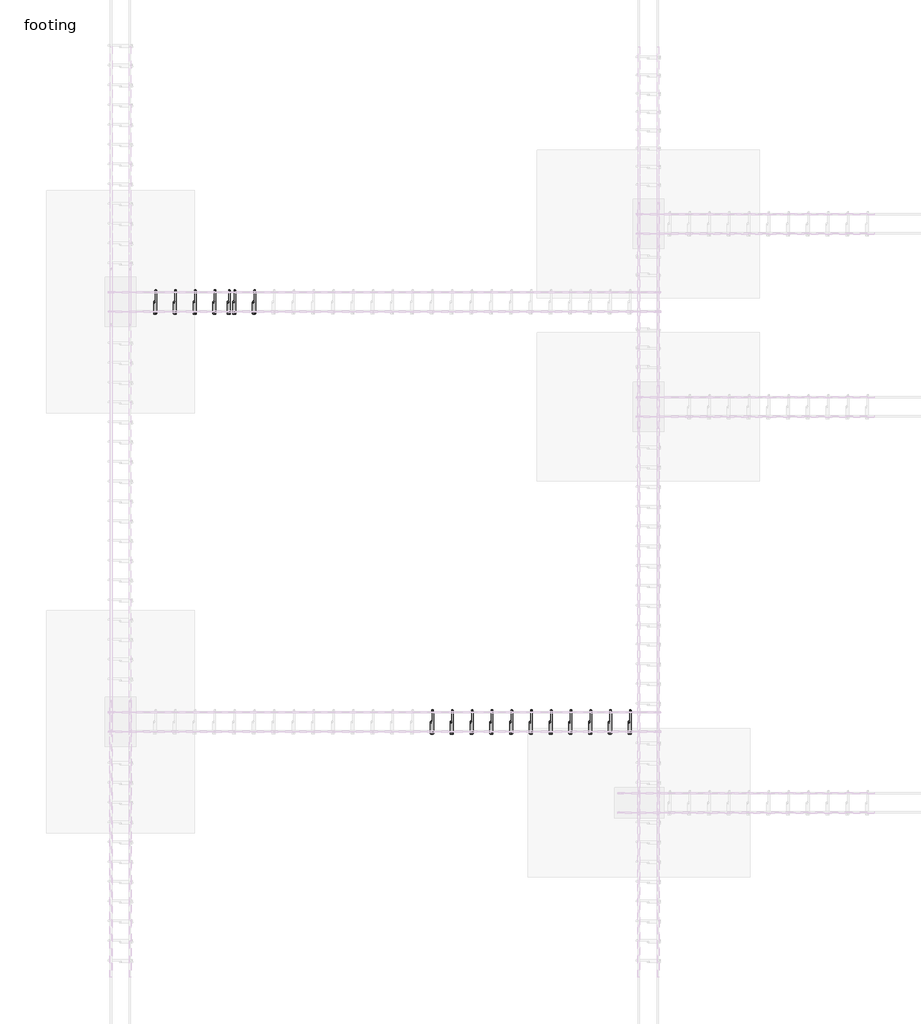
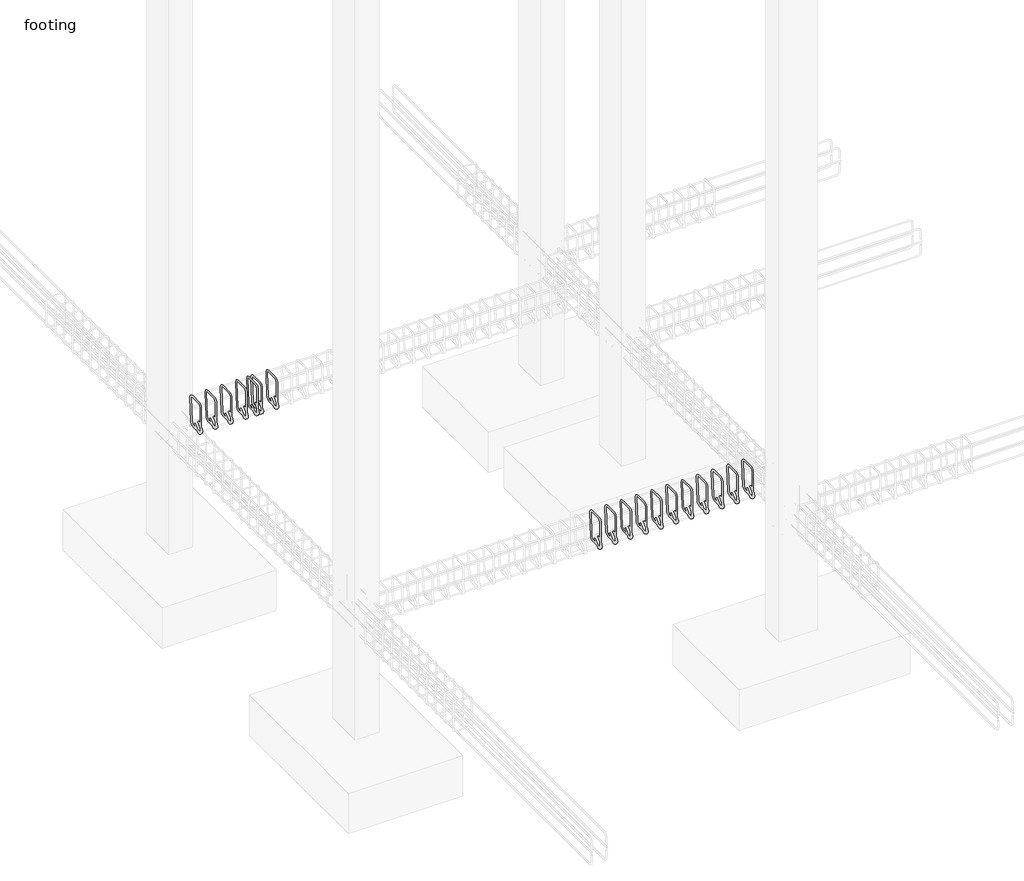
# One storey, part 7 of 21: 18 reinforcing bars.
"""IFC4 building model written with IfcOpenShell, lengths in millimetres."""

from ifc_helpers import new_model, si_unit, point, frame, origin, place, context, project, spatial, polyline, circle_curve, trimmed, segment, composite_curve, element, save
from ifc_brep_helpers import swept_disk

model = new_model("IFC4")

# Units and contexts
model_context = context("Model", 3, world=origin())
ifc_project = project(units=[si_unit("LENGTHUNIT", "METRE", prefix="MILLI")], contexts=[model_context])

# Site, building, storey
site = spatial("IfcSite", under=ifc_project)
building = spatial("IfcBuilding", under=site)
storey = spatial("IfcBuildingStorey", under=building, Name="footing", Elevation=-1524.0)

# Reinforcing bars
placement = place(None, origin())
element("IfcReinforcingBar", 1, at=placement, inside=storey, context=model_context, shape_type="SolidModel", body=[
    swept_disk(composite_curve([segment(polyline([(-9654.4883428, 4117.8887132, -310.8825168), (-9654.4883428, 4063.0237147, -365.7475153)]), True, "CONTINUOUS"), segment(trimmed(circle_curve(frame((-9654.4883428, 4040.5730744, -343.296875), z_axis=(-1.0, 0.0, 0.0), x_axis=(0.0, 22.450640299999577, -22.450640299999975)), 31.75), [point((-9654.4883428, 4063.0237147, -365.7475153))], [point((-9654.4883428, 4008.8230744, -343.296875))], True, "CARTESIAN"), True, "CONTINUOUS"), segment(polyline([(-9654.4883428, 4008.8230744, -343.296875), (-9654.4883428, 4008.8230744, -63.103125)]), True, "CONTINUOUS"), segment(trimmed(circle_curve(frame((-9654.4883428, 4040.5730744, -63.103125), z_axis=(-1.0, 0.0, 0.0), x_axis=(0.0, -31.75, 0.0)), 31.75), [point((-9654.4883428, 4008.8230744, -63.103125))], [point((-9654.4883428, 4040.5730744, -31.353125))], True, "CARTESIAN"), True, "CONTINUOUS"), segment(polyline([(-9654.4883428, 4040.5730744, -31.353125), (-9654.4883428, 4168.3668244, -31.353125)]), True, "CONTINUOUS"), segment(trimmed(circle_curve(frame((-9653.3159328, 4168.3668244, -63.0814712), z_axis=(-0.9993179916193466, 0.0, -0.03692629992126919), x_axis=(-1.1724099999992177, 0.0, 31.728346200000004)), 31.75), [point((-9654.4883428, 4168.3668244, -31.353125))], [point((-9653.3159328, 4200.1168244, -63.0814712))], True, "CARTESIAN"), True, "CONTINUOUS"), segment(polyline([(-9653.3159328, 4200.1168244, -63.0814712), (-9642.9607528, 4200.1168244, -343.3185288)]), True, "CONTINUOUS"), segment(trimmed(circle_curve(frame((-9642.9607528, 4168.3668244, -343.3185288), z_axis=(-0.9993179916193466, 0.0, -0.03692629992126919), x_axis=(0.0, 31.75, 0.0)), 31.75), [point((-9642.9607528, 4200.1168244, -343.3185288))], [point((-9641.7883428, 4168.3668244, -375.046875))], True, "CARTESIAN"), True, "CONTINUOUS"), segment(polyline([(-9641.7883428, 4168.3668244, -375.046875), (-9641.7883428, 4040.5730744, -375.046875)]), True, "CONTINUOUS"), segment(trimmed(circle_curve(frame((-9641.7883428, 4040.5730744, -343.296875), z_axis=(-1.0, 0.0, 0.0), x_axis=(0.0, 0.0, -31.75)), 31.75), [point((-9641.7883428, 4040.5730744, -375.046875))], [point((-9641.7883428, 4018.1224341, -320.8462347))], True, "CARTESIAN"), True, "CONTINUOUS"), segment(polyline([(-9641.7883428, 4018.1224341, -320.8462347), (-9641.7883428, 4072.9874326, -265.9812362)]), True, "CONTINUOUS")], self_intersect=False), 6.35),
])
element("IfcReinforcingBar", 2, at=placement, inside=storey, context=model_context, shape_type="SolidModel", body=[
    swept_disk(composite_curve([segment(polyline([(-9491.7883428, 4117.8887132, -310.8825168), (-9491.7883428, 4063.0237147, -365.7475153)]), True, "CONTINUOUS"), segment(trimmed(circle_curve(frame((-9491.7883428, 4040.5730744, -343.296875), z_axis=(-1.0, 0.0, 0.0), x_axis=(0.0, 22.450640299999577, -22.450640299999975)), 31.75), [point((-9491.7883428, 4063.0237147, -365.7475153))], [point((-9491.7883428, 4008.8230744, -343.296875))], True, "CARTESIAN"), True, "CONTINUOUS"), segment(polyline([(-9491.7883428, 4008.8230744, -343.296875), (-9491.7883428, 4008.8230744, -63.103125)]), True, "CONTINUOUS"), segment(trimmed(circle_curve(frame((-9491.7883428, 4040.5730744, -63.103125), z_axis=(-1.0, 0.0, 0.0), x_axis=(0.0, -31.75, 0.0)), 31.75), [point((-9491.7883428, 4008.8230744, -63.103125))], [point((-9491.7883428, 4040.5730744, -31.353125))], True, "CARTESIAN"), True, "CONTINUOUS"), segment(polyline([(-9491.7883428, 4040.5730744, -31.353125), (-9491.7883428, 4168.3668244, -31.353125)]), True, "CONTINUOUS"), segment(trimmed(circle_curve(frame((-9490.6159328, 4168.3668244, -63.0814712), z_axis=(-0.9993179916193466, 0.0, -0.03692629992126919), x_axis=(-1.1724100000010367, 0.0, 31.728346200000004)), 31.75), [point((-9491.7883428, 4168.3668244, -31.353125))], [point((-9490.6159328, 4200.1168244, -63.0814712))], True, "CARTESIAN"), True, "CONTINUOUS"), segment(polyline([(-9490.6159328, 4200.1168244, -63.0814712), (-9480.2607528, 4200.1168244, -343.3185288)]), True, "CONTINUOUS"), segment(trimmed(circle_curve(frame((-9480.2607528, 4168.3668244, -343.3185288), z_axis=(-0.9993179916193466, 0.0, -0.03692629992126919), x_axis=(0.0, 31.75, 0.0)), 31.75), [point((-9480.2607528, 4200.1168244, -343.3185288))], [point((-9479.0883428, 4168.3668244, -375.046875))], True, "CARTESIAN"), True, "CONTINUOUS"), segment(polyline([(-9479.0883428, 4168.3668244, -375.046875), (-9479.0883428, 4040.5730744, -375.046875)]), True, "CONTINUOUS"), segment(trimmed(circle_curve(frame((-9479.0883428, 4040.5730744, -343.296875), z_axis=(-1.0, 0.0, 0.0), x_axis=(0.0, 0.0, -31.75)), 31.75), [point((-9479.0883428, 4040.5730744, -375.046875))], [point((-9479.0883428, 4018.1224341, -320.8462347))], True, "CARTESIAN"), True, "CONTINUOUS"), segment(polyline([(-9479.0883428, 4018.1224341, -320.8462347), (-9479.0883428, 4072.9874326, -265.9812362)]), True, "CONTINUOUS")], self_intersect=False), 6.35),
])
element("IfcReinforcingBar", 3, at=placement, inside=storey, context=model_context, shape_type="SolidModel", body=[
    swept_disk(composite_curve([segment(polyline([(-9329.0883428, 4117.8887132, -310.8825168), (-9329.0883428, 4063.0237147, -365.7475153)]), True, "CONTINUOUS"), segment(trimmed(circle_curve(frame((-9329.0883428, 4040.5730744, -343.296875), z_axis=(-1.0, 0.0, 0.0), x_axis=(0.0, 22.450640299999577, -22.450640299999975)), 31.75), [point((-9329.0883428, 4063.0237147, -365.7475153))], [point((-9329.0883428, 4008.8230744, -343.296875))], True, "CARTESIAN"), True, "CONTINUOUS"), segment(polyline([(-9329.0883428, 4008.8230744, -343.296875), (-9329.0883428, 4008.8230744, -63.103125)]), True, "CONTINUOUS"), segment(trimmed(circle_curve(frame((-9329.0883428, 4040.5730744, -63.103125), z_axis=(-1.0, 0.0, 0.0), x_axis=(0.0, -31.75, 0.0)), 31.75), [point((-9329.0883428, 4008.8230744, -63.103125))], [point((-9329.0883428, 4040.5730744, -31.353125))], True, "CARTESIAN"), True, "CONTINUOUS"), segment(polyline([(-9329.0883428, 4040.5730744, -31.353125), (-9329.0883428, 4168.3668244, -31.353125)]), True, "CONTINUOUS"), segment(trimmed(circle_curve(frame((-9327.9159328, 4168.3668244, -63.0814712), z_axis=(-0.9993179916193466, 0.0, -0.03692629992126919), x_axis=(-1.1724099999992177, 0.0, 31.728346200000004)), 31.75), [point((-9329.0883428, 4168.3668244, -31.353125))], [point((-9327.9159328, 4200.1168244, -63.0814712))], True, "CARTESIAN"), True, "CONTINUOUS"), segment(polyline([(-9327.9159328, 4200.1168244, -63.0814712), (-9317.5607528, 4200.1168244, -343.3185288)]), True, "CONTINUOUS"), segment(trimmed(circle_curve(frame((-9317.5607528, 4168.3668244, -343.3185288), z_axis=(-0.9993179916193466, 0.0, -0.03692629992126919), x_axis=(0.0, 31.75, 0.0)), 31.75), [point((-9317.5607528, 4200.1168244, -343.3185288))], [point((-9316.3883428, 4168.3668244, -375.046875))], True, "CARTESIAN"), True, "CONTINUOUS"), segment(polyline([(-9316.3883428, 4168.3668244, -375.046875), (-9316.3883428, 4040.5730744, -375.046875)]), True, "CONTINUOUS"), segment(trimmed(circle_curve(frame((-9316.3883428, 4040.5730744, -343.296875), z_axis=(-1.0, 0.0, 0.0), x_axis=(0.0, 0.0, -31.75)), 31.75), [point((-9316.3883428, 4040.5730744, -375.046875))], [point((-9316.3883428, 4018.1224341, -320.8462347))], True, "CARTESIAN"), True, "CONTINUOUS"), segment(polyline([(-9316.3883428, 4018.1224341, -320.8462347), (-9316.3883428, 4072.9874326, -265.9812362)]), True, "CONTINUOUS")], self_intersect=False), 6.35),
])
element("IfcReinforcingBar", 4, at=placement, inside=storey, context=model_context, shape_type="SolidModel", body=[
    swept_disk(composite_curve([segment(polyline([(-9166.3883428, 4117.8887132, -310.8825168), (-9166.3883428, 4063.0237147, -365.7475153)]), True, "CONTINUOUS"), segment(trimmed(circle_curve(frame((-9166.3883428, 4040.5730744, -343.296875), z_axis=(-1.0, 0.0, 0.0), x_axis=(0.0, 22.450640299999577, -22.450640299999975)), 31.75), [point((-9166.3883428, 4063.0237147, -365.7475153))], [point((-9166.3883428, 4008.8230744, -343.296875))], True, "CARTESIAN"), True, "CONTINUOUS"), segment(polyline([(-9166.3883428, 4008.8230744, -343.296875), (-9166.3883428, 4008.8230744, -63.103125)]), True, "CONTINUOUS"), segment(trimmed(circle_curve(frame((-9166.3883428, 4040.5730744, -63.103125), z_axis=(-1.0, 0.0, 0.0), x_axis=(0.0, -31.75, 0.0)), 31.75), [point((-9166.3883428, 4008.8230744, -63.103125))], [point((-9166.3883428, 4040.5730744, -31.353125))], True, "CARTESIAN"), True, "CONTINUOUS"), segment(polyline([(-9166.3883428, 4040.5730744, -31.353125), (-9166.3883428, 4168.3668244, -31.353125)]), True, "CONTINUOUS"), segment(trimmed(circle_curve(frame((-9165.2159328, 4168.3668244, -63.0814712), z_axis=(-0.9993179916193466, 0.0, -0.03692629992126919), x_axis=(-1.1724100000010367, 0.0, 31.728346200000004)), 31.75), [point((-9166.3883428, 4168.3668244, -31.353125))], [point((-9165.2159328, 4200.1168244, -63.0814712))], True, "CARTESIAN"), True, "CONTINUOUS"), segment(polyline([(-9165.2159328, 4200.1168244, -63.0814712), (-9154.8607528, 4200.1168244, -343.3185288)]), True, "CONTINUOUS"), segment(trimmed(circle_curve(frame((-9154.8607528, 4168.3668244, -343.3185288), z_axis=(-0.9993179916193466, 0.0, -0.03692629992126919), x_axis=(0.0, 31.75, 0.0)), 31.75), [point((-9154.8607528, 4200.1168244, -343.3185288))], [point((-9153.6883428, 4168.3668244, -375.046875))], True, "CARTESIAN"), True, "CONTINUOUS"), segment(polyline([(-9153.6883428, 4168.3668244, -375.046875), (-9153.6883428, 4040.5730744, -375.046875)]), True, "CONTINUOUS"), segment(trimmed(circle_curve(frame((-9153.6883428, 4040.5730744, -343.296875), z_axis=(-1.0, 0.0, 0.0), x_axis=(0.0, 0.0, -31.75)), 31.75), [point((-9153.6883428, 4040.5730744, -375.046875))], [point((-9153.6883428, 4018.1224341, -320.8462347))], True, "CARTESIAN"), True, "CONTINUOUS"), segment(polyline([(-9153.6883428, 4018.1224341, -320.8462347), (-9153.6883428, 4072.9874326, -265.9812362)]), True, "CONTINUOUS")], self_intersect=False), 6.35),
])
element("IfcReinforcingBar", 5, at=placement, inside=storey, context=model_context, shape_type="SolidModel", body=[
    swept_disk(composite_curve([segment(polyline([(-9003.6883428, 4117.8887132, -310.8825168), (-9003.6883428, 4063.0237147, -365.7475153)]), True, "CONTINUOUS"), segment(trimmed(circle_curve(frame((-9003.6883428, 4040.5730744, -343.296875), z_axis=(-1.0, 0.0, 0.0), x_axis=(0.0, 22.450640299999577, -22.450640299999975)), 31.75), [point((-9003.6883428, 4063.0237147, -365.7475153))], [point((-9003.6883428, 4008.8230744, -343.296875))], True, "CARTESIAN"), True, "CONTINUOUS"), segment(polyline([(-9003.6883428, 4008.8230744, -343.296875), (-9003.6883428, 4008.8230744, -63.103125)]), True, "CONTINUOUS"), segment(trimmed(circle_curve(frame((-9003.6883428, 4040.5730744, -63.103125), z_axis=(-1.0, 0.0, 0.0), x_axis=(0.0, -31.75, 0.0)), 31.75), [point((-9003.6883428, 4008.8230744, -63.103125))], [point((-9003.6883428, 4040.5730744, -31.353125))], True, "CARTESIAN"), True, "CONTINUOUS"), segment(polyline([(-9003.6883428, 4040.5730744, -31.353125), (-9003.6883428, 4168.3668244, -31.353125)]), True, "CONTINUOUS"), segment(trimmed(circle_curve(frame((-9002.5159328, 4168.3668244, -63.0814712), z_axis=(-0.9993179916193466, 0.0, -0.03692629992126919), x_axis=(-1.1724099999992177, 0.0, 31.728346200000004)), 31.75), [point((-9003.6883428, 4168.3668244, -31.353125))], [point((-9002.5159328, 4200.1168244, -63.0814712))], True, "CARTESIAN"), True, "CONTINUOUS"), segment(polyline([(-9002.5159328, 4200.1168244, -63.0814712), (-8992.1607528, 4200.1168244, -343.3185288)]), True, "CONTINUOUS"), segment(trimmed(circle_curve(frame((-8992.1607528, 4168.3668244, -343.3185288), z_axis=(-0.9993179916193466, 0.0, -0.03692629992126919), x_axis=(0.0, 31.75, 0.0)), 31.75), [point((-8992.1607528, 4200.1168244, -343.3185288))], [point((-8990.9883428, 4168.3668244, -375.046875))], True, "CARTESIAN"), True, "CONTINUOUS"), segment(polyline([(-8990.9883428, 4168.3668244, -375.046875), (-8990.9883428, 4040.5730744, -375.046875)]), True, "CONTINUOUS"), segment(trimmed(circle_curve(frame((-8990.9883428, 4040.5730744, -343.296875), z_axis=(-1.0, 0.0, 0.0), x_axis=(0.0, 0.0, -31.75)), 31.75), [point((-8990.9883428, 4040.5730744, -375.046875))], [point((-8990.9883428, 4018.1224341, -320.8462347))], True, "CARTESIAN"), True, "CONTINUOUS"), segment(polyline([(-8990.9883428, 4018.1224341, -320.8462347), (-8990.9883428, 4072.9874326, -265.9812362)]), True, "CONTINUOUS")], self_intersect=False), 6.35),
])
element("IfcReinforcingBar", 6, at=placement, inside=storey, context=model_context, shape_type="SolidModel", body=[
    swept_disk(composite_curve([segment(polyline([(-8840.9883428, 4117.8887132, -310.8825168), (-8840.9883428, 4063.0237147, -365.7475153)]), True, "CONTINUOUS"), segment(trimmed(circle_curve(frame((-8840.9883428, 4040.5730744, -343.296875), z_axis=(-1.0, 0.0, 0.0), x_axis=(0.0, 22.450640299999577, -22.450640299999975)), 31.75), [point((-8840.9883428, 4063.0237147, -365.7475153))], [point((-8840.9883428, 4008.8230744, -343.296875))], True, "CARTESIAN"), True, "CONTINUOUS"), segment(polyline([(-8840.9883428, 4008.8230744, -343.296875), (-8840.9883428, 4008.8230744, -63.103125)]), True, "CONTINUOUS"), segment(trimmed(circle_curve(frame((-8840.9883428, 4040.5730744, -63.103125), z_axis=(-1.0, 0.0, 0.0), x_axis=(0.0, -31.75, 0.0)), 31.75), [point((-8840.9883428, 4008.8230744, -63.103125))], [point((-8840.9883428, 4040.5730744, -31.353125))], True, "CARTESIAN"), True, "CONTINUOUS"), segment(polyline([(-8840.9883428, 4040.5730744, -31.353125), (-8840.9883428, 4168.3668244, -31.353125)]), True, "CONTINUOUS"), segment(trimmed(circle_curve(frame((-8839.8159328, 4168.3668244, -63.0814712), z_axis=(-0.9993179916193466, 0.0, -0.03692629992126919), x_axis=(-1.1724099999992177, 0.0, 31.728346200000004)), 31.75), [point((-8840.9883428, 4168.3668244, -31.353125))], [point((-8839.8159328, 4200.1168244, -63.0814712))], True, "CARTESIAN"), True, "CONTINUOUS"), segment(polyline([(-8839.8159328, 4200.1168244, -63.0814712), (-8829.4607528, 4200.1168244, -343.3185288)]), True, "CONTINUOUS"), segment(trimmed(circle_curve(frame((-8829.4607528, 4168.3668244, -343.3185288), z_axis=(-0.9993179916193466, 0.0, -0.03692629992126919), x_axis=(0.0, 31.75, 0.0)), 31.75), [point((-8829.4607528, 4200.1168244, -343.3185288))], [point((-8828.2883428, 4168.3668244, -375.046875))], True, "CARTESIAN"), True, "CONTINUOUS"), segment(polyline([(-8828.2883428, 4168.3668244, -375.046875), (-8828.2883428, 4040.5730744, -375.046875)]), True, "CONTINUOUS"), segment(trimmed(circle_curve(frame((-8828.2883428, 4040.5730744, -343.296875), z_axis=(-1.0, 0.0, 0.0), x_axis=(0.0, 0.0, -31.75)), 31.75), [point((-8828.2883428, 4040.5730744, -375.046875))], [point((-8828.2883428, 4018.1224341, -320.8462347))], True, "CARTESIAN"), True, "CONTINUOUS"), segment(polyline([(-8828.2883428, 4018.1224341, -320.8462347), (-8828.2883428, 4072.9874326, -265.9812362)]), True, "CONTINUOUS")], self_intersect=False), 6.35),
])
element("IfcReinforcingBar", 7, at=placement, inside=storey, context=model_context, shape_type="SolidModel", body=[
    swept_disk(composite_curve([segment(polyline([(-8678.2883428, 4117.8887132, -310.8825168), (-8678.2883428, 4063.0237147, -365.7475153)]), True, "CONTINUOUS"), segment(trimmed(circle_curve(frame((-8678.2883428, 4040.5730744, -343.296875), z_axis=(-1.0, 0.0, 0.0), x_axis=(0.0, 22.450640299999577, -22.450640299999975)), 31.75), [point((-8678.2883428, 4063.0237147, -365.7475153))], [point((-8678.2883428, 4008.8230744, -343.296875))], True, "CARTESIAN"), True, "CONTINUOUS"), segment(polyline([(-8678.2883428, 4008.8230744, -343.296875), (-8678.2883428, 4008.8230744, -63.103125)]), True, "CONTINUOUS"), segment(trimmed(circle_curve(frame((-8678.2883428, 4040.5730744, -63.103125), z_axis=(-1.0, 0.0, 0.0), x_axis=(0.0, -31.75, 0.0)), 31.75), [point((-8678.2883428, 4008.8230744, -63.103125))], [point((-8678.2883428, 4040.5730744, -31.353125))], True, "CARTESIAN"), True, "CONTINUOUS"), segment(polyline([(-8678.2883428, 4040.5730744, -31.353125), (-8678.2883428, 4168.3668244, -31.353125)]), True, "CONTINUOUS"), segment(trimmed(circle_curve(frame((-8677.1159328, 4168.3668244, -63.0814712), z_axis=(-0.9993179916193466, 0.0, -0.03692629992126919), x_axis=(-1.1724100000010367, 0.0, 31.728346200000004)), 31.75), [point((-8678.2883428, 4168.3668244, -31.353125))], [point((-8677.1159328, 4200.1168244, -63.0814712))], True, "CARTESIAN"), True, "CONTINUOUS"), segment(polyline([(-8677.1159328, 4200.1168244, -63.0814712), (-8666.7607528, 4200.1168244, -343.3185288)]), True, "CONTINUOUS"), segment(trimmed(circle_curve(frame((-8666.7607528, 4168.3668244, -343.3185288), z_axis=(-0.9993179916193466, 0.0, -0.03692629992126919), x_axis=(0.0, 31.75, 0.0)), 31.75), [point((-8666.7607528, 4200.1168244, -343.3185288))], [point((-8665.5883428, 4168.3668244, -375.046875))], True, "CARTESIAN"), True, "CONTINUOUS"), segment(polyline([(-8665.5883428, 4168.3668244, -375.046875), (-8665.5883428, 4040.5730744, -375.046875)]), True, "CONTINUOUS"), segment(trimmed(circle_curve(frame((-8665.5883428, 4040.5730744, -343.296875), z_axis=(-1.0, 0.0, 0.0), x_axis=(0.0, 0.0, -31.75)), 31.75), [point((-8665.5883428, 4040.5730744, -375.046875))], [point((-8665.5883428, 4018.1224341, -320.8462347))], True, "CARTESIAN"), True, "CONTINUOUS"), segment(polyline([(-8665.5883428, 4018.1224341, -320.8462347), (-8665.5883428, 4072.9874326, -265.9812362)]), True, "CONTINUOUS")], self_intersect=False), 6.35),
])
element("IfcReinforcingBar", 8, at=placement, inside=storey, context=model_context, shape_type="SolidModel", body=[
    swept_disk(composite_curve([segment(polyline([(-8515.5883428, 4117.8887132, -310.8825168), (-8515.5883428, 4063.0237147, -365.7475153)]), True, "CONTINUOUS"), segment(trimmed(circle_curve(frame((-8515.5883428, 4040.5730744, -343.296875), z_axis=(-1.0, 0.0, 0.0), x_axis=(0.0, 22.450640299999577, -22.450640299999975)), 31.75), [point((-8515.5883428, 4063.0237147, -365.7475153))], [point((-8515.5883428, 4008.8230744, -343.296875))], True, "CARTESIAN"), True, "CONTINUOUS"), segment(polyline([(-8515.5883428, 4008.8230744, -343.296875), (-8515.5883428, 4008.8230744, -63.103125)]), True, "CONTINUOUS"), segment(trimmed(circle_curve(frame((-8515.5883428, 4040.5730744, -63.103125), z_axis=(-1.0, 0.0, 0.0), x_axis=(0.0, -31.75, 0.0)), 31.75), [point((-8515.5883428, 4008.8230744, -63.103125))], [point((-8515.5883428, 4040.5730744, -31.353125))], True, "CARTESIAN"), True, "CONTINUOUS"), segment(polyline([(-8515.5883428, 4040.5730744, -31.353125), (-8515.5883428, 4168.3668244, -31.353125)]), True, "CONTINUOUS"), segment(trimmed(circle_curve(frame((-8514.4159328, 4168.3668244, -63.0814712), z_axis=(-0.9993179916193466, 0.0, -0.03692629992126919), x_axis=(-1.1724099999992177, 0.0, 31.728346200000004)), 31.75), [point((-8515.5883428, 4168.3668244, -31.353125))], [point((-8514.4159328, 4200.1168244, -63.0814712))], True, "CARTESIAN"), True, "CONTINUOUS"), segment(polyline([(-8514.4159328, 4200.1168244, -63.0814712), (-8504.0607528, 4200.1168244, -343.3185288)]), True, "CONTINUOUS"), segment(trimmed(circle_curve(frame((-8504.0607528, 4168.3668244, -343.3185288), z_axis=(-0.9993179916193466, 0.0, -0.03692629992126919), x_axis=(0.0, 31.75, 0.0)), 31.75), [point((-8504.0607528, 4200.1168244, -343.3185288))], [point((-8502.8883428, 4168.3668244, -375.046875))], True, "CARTESIAN"), True, "CONTINUOUS"), segment(polyline([(-8502.8883428, 4168.3668244, -375.046875), (-8502.8883428, 4040.5730744, -375.046875)]), True, "CONTINUOUS"), segment(trimmed(circle_curve(frame((-8502.8883428, 4040.5730744, -343.296875), z_axis=(-1.0, 0.0, 0.0), x_axis=(0.0, 0.0, -31.75)), 31.75), [point((-8502.8883428, 4040.5730744, -375.046875))], [point((-8502.8883428, 4018.1224341, -320.8462347))], True, "CARTESIAN"), True, "CONTINUOUS"), segment(polyline([(-8502.8883428, 4018.1224341, -320.8462347), (-8502.8883428, 4072.9874326, -265.9812362)]), True, "CONTINUOUS")], self_intersect=False), 6.35),
])
element("IfcReinforcingBar", 9, at=placement, inside=storey, context=model_context, shape_type="SolidModel", body=[
    swept_disk(composite_curve([segment(polyline([(-8352.8883428, 4117.8887132, -310.8825168), (-8352.8883428, 4063.0237147, -365.7475153)]), True, "CONTINUOUS"), segment(trimmed(circle_curve(frame((-8352.8883428, 4040.5730744, -343.296875), z_axis=(-1.0, 0.0, 0.0), x_axis=(0.0, 22.450640299999577, -22.450640299999975)), 31.75), [point((-8352.8883428, 4063.0237147, -365.7475153))], [point((-8352.8883428, 4008.8230744, -343.296875))], True, "CARTESIAN"), True, "CONTINUOUS"), segment(polyline([(-8352.8883428, 4008.8230744, -343.296875), (-8352.8883428, 4008.8230744, -63.103125)]), True, "CONTINUOUS"), segment(trimmed(circle_curve(frame((-8352.8883428, 4040.5730744, -63.103125), z_axis=(-1.0, 0.0, 0.0), x_axis=(0.0, -31.75, 0.0)), 31.75), [point((-8352.8883428, 4008.8230744, -63.103125))], [point((-8352.8883428, 4040.5730744, -31.353125))], True, "CARTESIAN"), True, "CONTINUOUS"), segment(polyline([(-8352.8883428, 4040.5730744, -31.353125), (-8352.8883428, 4168.3668244, -31.353125)]), True, "CONTINUOUS"), segment(trimmed(circle_curve(frame((-8351.7159328, 4168.3668244, -63.0814712), z_axis=(-0.9993179916193466, 0.0, -0.03692629992126919), x_axis=(-1.1724100000010367, 0.0, 31.728346200000004)), 31.75), [point((-8352.8883428, 4168.3668244, -31.353125))], [point((-8351.7159328, 4200.1168244, -63.0814712))], True, "CARTESIAN"), True, "CONTINUOUS"), segment(polyline([(-8351.7159328, 4200.1168244, -63.0814712), (-8341.3607528, 4200.1168244, -343.3185288)]), True, "CONTINUOUS"), segment(trimmed(circle_curve(frame((-8341.3607528, 4168.3668244, -343.3185288), z_axis=(-0.9993179916193466, 0.0, -0.03692629992126919), x_axis=(0.0, 31.75, 0.0)), 31.75), [point((-8341.3607528, 4200.1168244, -343.3185288))], [point((-8340.1883428, 4168.3668244, -375.046875))], True, "CARTESIAN"), True, "CONTINUOUS"), segment(polyline([(-8340.1883428, 4168.3668244, -375.046875), (-8340.1883428, 4040.5730744, -375.046875)]), True, "CONTINUOUS"), segment(trimmed(circle_curve(frame((-8340.1883428, 4040.5730744, -343.296875), z_axis=(-1.0, 0.0, 0.0), x_axis=(0.0, 0.0, -31.75)), 31.75), [point((-8340.1883428, 4040.5730744, -375.046875))], [point((-8340.1883428, 4018.1224341, -320.8462347))], True, "CARTESIAN"), True, "CONTINUOUS"), segment(polyline([(-8340.1883428, 4018.1224341, -320.8462347), (-8340.1883428, 4072.9874326, -265.9812362)]), True, "CONTINUOUS")], self_intersect=False), 6.35),
])
element("IfcReinforcingBar", 10, at=placement, inside=storey, context=model_context, shape_type="SolidModel", body=[
    swept_disk(composite_curve([segment(polyline([(-8190.1883428, 4117.8887132, -310.8825168), (-8190.1883428, 4063.0237147, -365.7475153)]), True, "CONTINUOUS"), segment(trimmed(circle_curve(frame((-8190.1883428, 4040.5730744, -343.296875), z_axis=(-1.0, 0.0, 0.0), x_axis=(0.0, 22.450640299999577, -22.450640299999975)), 31.75), [point((-8190.1883428, 4063.0237147, -365.7475153))], [point((-8190.1883428, 4008.8230744, -343.296875))], True, "CARTESIAN"), True, "CONTINUOUS"), segment(polyline([(-8190.1883428, 4008.8230744, -343.296875), (-8190.1883428, 4008.8230744, -63.103125)]), True, "CONTINUOUS"), segment(trimmed(circle_curve(frame((-8190.1883428, 4040.5730744, -63.103125), z_axis=(-1.0, 0.0, 0.0), x_axis=(0.0, -31.75, 0.0)), 31.75), [point((-8190.1883428, 4008.8230744, -63.103125))], [point((-8190.1883428, 4040.5730744, -31.353125))], True, "CARTESIAN"), True, "CONTINUOUS"), segment(polyline([(-8190.1883428, 4040.5730744, -31.353125), (-8190.1883428, 4168.3668244, -31.353125)]), True, "CONTINUOUS"), segment(trimmed(circle_curve(frame((-8189.0159328, 4168.3668244, -63.0814712), z_axis=(-0.9993179916193466, 0.0, -0.03692629992126919), x_axis=(-1.1724100000001272, 0.0, 31.728346200000004)), 31.75), [point((-8190.1883428, 4168.3668244, -31.353125))], [point((-8189.0159328, 4200.1168244, -63.0814712))], True, "CARTESIAN"), True, "CONTINUOUS"), segment(polyline([(-8189.0159328, 4200.1168244, -63.0814712), (-8178.6607528, 4200.1168244, -343.3185288)]), True, "CONTINUOUS"), segment(trimmed(circle_curve(frame((-8178.6607528, 4168.3668244, -343.3185288), z_axis=(-0.9993179916193466, 0.0, -0.03692629992126919), x_axis=(0.0, 31.75, 0.0)), 31.75), [point((-8178.6607528, 4200.1168244, -343.3185288))], [point((-8177.4883428, 4168.3668244, -375.046875))], True, "CARTESIAN"), True, "CONTINUOUS"), segment(polyline([(-8177.4883428, 4168.3668244, -375.046875), (-8177.4883428, 4040.5730744, -375.046875)]), True, "CONTINUOUS"), segment(trimmed(circle_curve(frame((-8177.4883428, 4040.5730744, -343.296875), z_axis=(-1.0, 0.0, 0.0), x_axis=(0.0, 0.0, -31.75)), 31.75), [point((-8177.4883428, 4040.5730744, -375.046875))], [point((-8177.4883428, 4018.1224341, -320.8462347))], True, "CARTESIAN"), True, "CONTINUOUS"), segment(polyline([(-8177.4883428, 4018.1224341, -320.8462347), (-8177.4883428, 4072.9874326, -265.9812362)]), True, "CONTINUOUS")], self_intersect=False), 6.35),
])
element("IfcReinforcingBar", 11, at=placement, inside=storey, context=model_context, shape_type="SolidModel", body=[
    swept_disk(composite_curve([segment(polyline([(-11932.2883428, 7572.2887132, -310.8825168), (-11932.2883428, 7517.4237147, -365.7475153)]), True, "CONTINUOUS"), segment(trimmed(circle_curve(frame((-11932.2883428, 7494.9730744, -343.296875), z_axis=(-1.0, 0.0, 0.0), x_axis=(0.0, 22.450640300000487, -22.450640299999975)), 31.75), [point((-11932.2883428, 7517.4237147, -365.7475153))], [point((-11932.2883428, 7463.2230744, -343.296875))], True, "CARTESIAN"), True, "CONTINUOUS"), segment(polyline([(-11932.2883428, 7463.2230744, -343.296875), (-11932.2883428, 7463.2230744, -63.103125)]), True, "CONTINUOUS"), segment(trimmed(circle_curve(frame((-11932.2883428, 7494.9730744, -63.103125), z_axis=(-1.0, 0.0, 0.0), x_axis=(0.0, -31.75, 0.0)), 31.75), [point((-11932.2883428, 7463.2230744, -63.103125))], [point((-11932.2883428, 7494.9730744, -31.353125))], True, "CARTESIAN"), True, "CONTINUOUS"), segment(polyline([(-11932.2883428, 7494.9730744, -31.353125), (-11932.2883428, 7622.7668244, -31.353125)]), True, "CONTINUOUS"), segment(trimmed(circle_curve(frame((-11931.1159328, 7622.7668244, -63.0814712), z_axis=(-0.9993179916193466, 0.0, -0.03692629992126919), x_axis=(-1.1724100000010367, 0.0, 31.728346200000004)), 31.75), [point((-11932.2883428, 7622.7668244, -31.353125))], [point((-11931.1159328, 7654.5168244, -63.0814712))], True, "CARTESIAN"), True, "CONTINUOUS"), segment(polyline([(-11931.1159328, 7654.5168244, -63.0814712), (-11920.7607528, 7654.5168244, -343.3185288)]), True, "CONTINUOUS"), segment(trimmed(circle_curve(frame((-11920.7607528, 7622.7668244, -343.3185288), z_axis=(-0.9993179916193466, 0.0, -0.03692629992126919), x_axis=(0.0, 31.75, 0.0)), 31.75), [point((-11920.7607528, 7654.5168244, -343.3185288))], [point((-11919.5883428, 7622.7668244, -375.046875))], True, "CARTESIAN"), True, "CONTINUOUS"), segment(polyline([(-11919.5883428, 7622.7668244, -375.046875), (-11919.5883428, 7494.9730744, -375.046875)]), True, "CONTINUOUS"), segment(trimmed(circle_curve(frame((-11919.5883428, 7494.9730744, -343.296875), z_axis=(-1.0, 0.0, 0.0), x_axis=(0.0, 0.0, -31.75)), 31.75), [point((-11919.5883428, 7494.9730744, -375.046875))], [point((-11919.5883428, 7472.5224341, -320.8462347))], True, "CARTESIAN"), True, "CONTINUOUS"), segment(polyline([(-11919.5883428, 7472.5224341, -320.8462347), (-11919.5883428, 7527.3874326, -265.9812362)]), True, "CONTINUOUS")], self_intersect=False), 6.35),
])
element("IfcReinforcingBar", 12, at=placement, inside=storey, context=model_context, shape_type="SolidModel", body=[
    swept_disk(composite_curve([segment(polyline([(-11769.5883428, 7572.2887132, -310.8825168), (-11769.5883428, 7517.4237147, -365.7475153)]), True, "CONTINUOUS"), segment(trimmed(circle_curve(frame((-11769.5883428, 7494.9730744, -343.296875), z_axis=(-1.0, 0.0, 0.0), x_axis=(0.0, 22.450640300000487, -22.450640299999975)), 31.75), [point((-11769.5883428, 7517.4237147, -365.7475153))], [point((-11769.5883428, 7463.2230744, -343.296875))], True, "CARTESIAN"), True, "CONTINUOUS"), segment(polyline([(-11769.5883428, 7463.2230744, -343.296875), (-11769.5883428, 7463.2230744, -63.103125)]), True, "CONTINUOUS"), segment(trimmed(circle_curve(frame((-11769.5883428, 7494.9730744, -63.103125), z_axis=(-1.0, 0.0, 0.0), x_axis=(0.0, -31.75, 0.0)), 31.75), [point((-11769.5883428, 7463.2230744, -63.103125))], [point((-11769.5883428, 7494.9730744, -31.353125))], True, "CARTESIAN"), True, "CONTINUOUS"), segment(polyline([(-11769.5883428, 7494.9730744, -31.353125), (-11769.5883428, 7622.7668244, -31.353125)]), True, "CONTINUOUS"), segment(trimmed(circle_curve(frame((-11768.4159328, 7622.7668244, -63.0814712), z_axis=(-0.9993179916193466, 0.0, -0.03692629992126919), x_axis=(-1.1724099999992177, 0.0, 31.728346200000004)), 31.75), [point((-11769.5883428, 7622.7668244, -31.353125))], [point((-11768.4159328, 7654.5168244, -63.0814712))], True, "CARTESIAN"), True, "CONTINUOUS"), segment(polyline([(-11768.4159328, 7654.5168244, -63.0814712), (-11758.0607528, 7654.5168244, -343.3185288)]), True, "CONTINUOUS"), segment(trimmed(circle_curve(frame((-11758.0607528, 7622.7668244, -343.3185288), z_axis=(-0.9993179916193466, 0.0, -0.03692629992126919), x_axis=(0.0, 31.75, 0.0)), 31.75), [point((-11758.0607528, 7654.5168244, -343.3185288))], [point((-11756.8883428, 7622.7668244, -375.046875))], True, "CARTESIAN"), True, "CONTINUOUS"), segment(polyline([(-11756.8883428, 7622.7668244, -375.046875), (-11756.8883428, 7494.9730744, -375.046875)]), True, "CONTINUOUS"), segment(trimmed(circle_curve(frame((-11756.8883428, 7494.9730744, -343.296875), z_axis=(-1.0, 0.0, 0.0), x_axis=(0.0, 0.0, -31.75)), 31.75), [point((-11756.8883428, 7494.9730744, -375.046875))], [point((-11756.8883428, 7472.5224341, -320.8462347))], True, "CARTESIAN"), True, "CONTINUOUS"), segment(polyline([(-11756.8883428, 7472.5224341, -320.8462347), (-11756.8883428, 7527.3874326, -265.9812362)]), True, "CONTINUOUS")], self_intersect=False), 6.35),
])
element("IfcReinforcingBar", 13, at=placement, inside=storey, context=model_context, shape_type="SolidModel", body=[
    swept_disk(composite_curve([segment(polyline([(-11606.8883428, 7572.2887132, -310.8825168), (-11606.8883428, 7517.4237147, -365.7475153)]), True, "CONTINUOUS"), segment(trimmed(circle_curve(frame((-11606.8883428, 7494.9730744, -343.296875), z_axis=(-1.0, 0.0, 0.0), x_axis=(0.0, 22.450640300000487, -22.450640299999975)), 31.75), [point((-11606.8883428, 7517.4237147, -365.7475153))], [point((-11606.8883428, 7463.2230744, -343.296875))], True, "CARTESIAN"), True, "CONTINUOUS"), segment(polyline([(-11606.8883428, 7463.2230744, -343.296875), (-11606.8883428, 7463.2230744, -63.103125)]), True, "CONTINUOUS"), segment(trimmed(circle_curve(frame((-11606.8883428, 7494.9730744, -63.103125), z_axis=(-1.0, 0.0, 0.0), x_axis=(0.0, -31.75, 0.0)), 31.75), [point((-11606.8883428, 7463.2230744, -63.103125))], [point((-11606.8883428, 7494.9730744, -31.353125))], True, "CARTESIAN"), True, "CONTINUOUS"), segment(polyline([(-11606.8883428, 7494.9730744, -31.353125), (-11606.8883428, 7622.7668244, -31.353125)]), True, "CONTINUOUS"), segment(trimmed(circle_curve(frame((-11605.7159328, 7622.7668244, -63.0814712), z_axis=(-0.9993179916193466, 0.0, -0.03692629992126919), x_axis=(-1.1724100000010367, 0.0, 31.728346200000004)), 31.75), [point((-11606.8883428, 7622.7668244, -31.353125))], [point((-11605.7159328, 7654.5168244, -63.0814712))], True, "CARTESIAN"), True, "CONTINUOUS"), segment(polyline([(-11605.7159328, 7654.5168244, -63.0814712), (-11595.3607528, 7654.5168244, -343.3185288)]), True, "CONTINUOUS"), segment(trimmed(circle_curve(frame((-11595.3607528, 7622.7668244, -343.3185288), z_axis=(-0.9993179916193466, 0.0, -0.03692629992126919), x_axis=(0.0, 31.75, 0.0)), 31.75), [point((-11595.3607528, 7654.5168244, -343.3185288))], [point((-11594.1883428, 7622.7668244, -375.046875))], True, "CARTESIAN"), True, "CONTINUOUS"), segment(polyline([(-11594.1883428, 7622.7668244, -375.046875), (-11594.1883428, 7494.9730744, -375.046875)]), True, "CONTINUOUS"), segment(trimmed(circle_curve(frame((-11594.1883428, 7494.9730744, -343.296875), z_axis=(-1.0, 0.0, 0.0), x_axis=(0.0, 0.0, -31.75)), 31.75), [point((-11594.1883428, 7494.9730744, -375.046875))], [point((-11594.1883428, 7472.5224341, -320.8462347))], True, "CARTESIAN"), True, "CONTINUOUS"), segment(polyline([(-11594.1883428, 7472.5224341, -320.8462347), (-11594.1883428, 7527.3874326, -265.9812362)]), True, "CONTINUOUS")], self_intersect=False), 6.35),
])
element("IfcReinforcingBar", 14, at=placement, inside=storey, context=model_context, shape_type="SolidModel", body=[
    swept_disk(composite_curve([segment(polyline([(-11444.1883428, 7572.2887132, -310.8825168), (-11444.1883428, 7517.4237147, -365.7475153)]), True, "CONTINUOUS"), segment(trimmed(circle_curve(frame((-11444.1883428, 7494.9730744, -343.296875), z_axis=(-1.0, 0.0, 0.0), x_axis=(0.0, 22.450640300000487, -22.450640299999975)), 31.75), [point((-11444.1883428, 7517.4237147, -365.7475153))], [point((-11444.1883428, 7463.2230744, -343.296875))], True, "CARTESIAN"), True, "CONTINUOUS"), segment(polyline([(-11444.1883428, 7463.2230744, -343.296875), (-11444.1883428, 7463.2230744, -63.103125)]), True, "CONTINUOUS"), segment(trimmed(circle_curve(frame((-11444.1883428, 7494.9730744, -63.103125), z_axis=(-1.0, 0.0, 0.0), x_axis=(0.0, -31.75, 0.0)), 31.75), [point((-11444.1883428, 7463.2230744, -63.103125))], [point((-11444.1883428, 7494.9730744, -31.353125))], True, "CARTESIAN"), True, "CONTINUOUS"), segment(polyline([(-11444.1883428, 7494.9730744, -31.353125), (-11444.1883428, 7622.7668244, -31.353125)]), True, "CONTINUOUS"), segment(trimmed(circle_curve(frame((-11443.0159328, 7622.7668244, -63.0814712), z_axis=(-0.9993179916193466, 0.0, -0.03692629992126919), x_axis=(-1.1724099999992177, 0.0, 31.728346200000004)), 31.75), [point((-11444.1883428, 7622.7668244, -31.353125))], [point((-11443.0159328, 7654.5168244, -63.0814712))], True, "CARTESIAN"), True, "CONTINUOUS"), segment(polyline([(-11443.0159328, 7654.5168244, -63.0814712), (-11432.6607528, 7654.5168244, -343.3185288)]), True, "CONTINUOUS"), segment(trimmed(circle_curve(frame((-11432.6607528, 7622.7668244, -343.3185288), z_axis=(-0.9993179916193466, 0.0, -0.03692629992126919), x_axis=(0.0, 31.75, 0.0)), 31.75), [point((-11432.6607528, 7654.5168244, -343.3185288))], [point((-11431.4883428, 7622.7668244, -375.046875))], True, "CARTESIAN"), True, "CONTINUOUS"), segment(polyline([(-11431.4883428, 7622.7668244, -375.046875), (-11431.4883428, 7494.9730744, -375.046875)]), True, "CONTINUOUS"), segment(trimmed(circle_curve(frame((-11431.4883428, 7494.9730744, -343.296875), z_axis=(-1.0, 0.0, 0.0), x_axis=(0.0, 0.0, -31.75)), 31.75), [point((-11431.4883428, 7494.9730744, -375.046875))], [point((-11431.4883428, 7472.5224341, -320.8462347))], True, "CARTESIAN"), True, "CONTINUOUS"), segment(polyline([(-11431.4883428, 7472.5224341, -320.8462347), (-11431.4883428, 7527.3874326, -265.9812362)]), True, "CONTINUOUS")], self_intersect=False), 6.35),
])
element("IfcReinforcingBar", 15, at=placement, inside=storey, context=model_context, shape_type="SolidModel", body=[
    swept_disk(composite_curve([segment(polyline([(-11326.2490423, 7572.2887132, -310.8825168), (-11326.2490423, 7517.4237147, -365.7475153)]), True, "CONTINUOUS"), segment(trimmed(circle_curve(frame((-11326.2490423, 7494.9730744, -343.296875), z_axis=(-1.0, 0.0, 0.0), x_axis=(0.0, 22.450640300000487, -22.450640299999975)), 31.75), [point((-11326.2490423, 7517.4237147, -365.7475153))], [point((-11326.2490423, 7463.2230744, -343.296875))], True, "CARTESIAN"), True, "CONTINUOUS"), segment(polyline([(-11326.2490423, 7463.2230744, -343.296875), (-11326.2490423, 7463.2230744, -63.103125)]), True, "CONTINUOUS"), segment(trimmed(circle_curve(frame((-11326.2490423, 7494.9730744, -63.103125), z_axis=(-1.0, 0.0, 0.0), x_axis=(0.0, -31.75, 0.0)), 31.75), [point((-11326.2490423, 7463.2230744, -63.103125))], [point((-11326.2490423, 7494.9730744, -31.353125))], True, "CARTESIAN"), True, "CONTINUOUS"), segment(polyline([(-11326.2490423, 7494.9730744, -31.353125), (-11326.2490423, 7622.7668244, -31.353125)]), True, "CONTINUOUS"), segment(trimmed(circle_curve(frame((-11325.0766322, 7622.7668244, -63.0814712), z_axis=(-0.9993179916193466, 0.0, -0.03692629992126919), x_axis=(-1.1724100999999791, 0.0, 31.728346200000004)), 31.75), [point((-11326.2490423, 7622.7668244, -31.353125))], [point((-11325.0766322, 7654.5168244, -63.0814712))], True, "CARTESIAN"), True, "CONTINUOUS"), segment(polyline([(-11325.0766322, 7654.5168244, -63.0814712), (-11314.7214523, 7654.5168244, -343.3185288)]), True, "CONTINUOUS"), segment(trimmed(circle_curve(frame((-11314.7214523, 7622.7668244, -343.3185288), z_axis=(-0.9993179916193466, 0.0, -0.03692629992126919), x_axis=(0.0, 31.75, 0.0)), 31.75), [point((-11314.7214523, 7654.5168244, -343.3185288))], [point((-11313.5490423, 7622.7668244, -375.046875))], True, "CARTESIAN"), True, "CONTINUOUS"), segment(polyline([(-11313.5490423, 7622.7668244, -375.046875), (-11313.5490423, 7494.9730744, -375.046875)]), True, "CONTINUOUS"), segment(trimmed(circle_curve(frame((-11313.5490423, 7494.9730744, -343.296875), z_axis=(-1.0, 0.0, 0.0), x_axis=(0.0, 0.0, -31.75)), 31.75), [point((-11313.5490423, 7494.9730744, -375.046875))], [point((-11313.5490423, 7472.5224341, -320.8462347))], True, "CARTESIAN"), True, "CONTINUOUS"), segment(polyline([(-11313.5490423, 7472.5224341, -320.8462347), (-11313.5490423, 7527.3874326, -265.9812362)]), True, "CONTINUOUS")], self_intersect=False), 6.35),
])
element("IfcReinforcingBar", 16, at=placement, inside=storey, context=model_context, shape_type="SolidModel", body=[
    swept_disk(composite_curve([segment(polyline([(-11281.4883428, 7572.2887132, -310.8825168), (-11281.4883428, 7517.4237147, -365.7475153)]), True, "CONTINUOUS"), segment(trimmed(circle_curve(frame((-11281.4883428, 7494.9730744, -343.296875), z_axis=(-1.0, 0.0, 0.0), x_axis=(0.0, 22.450640300000487, -22.450640299999975)), 31.75), [point((-11281.4883428, 7517.4237147, -365.7475153))], [point((-11281.4883428, 7463.2230744, -343.296875))], True, "CARTESIAN"), True, "CONTINUOUS"), segment(polyline([(-11281.4883428, 7463.2230744, -343.296875), (-11281.4883428, 7463.2230744, -63.103125)]), True, "CONTINUOUS"), segment(trimmed(circle_curve(frame((-11281.4883428, 7494.9730744, -63.103125), z_axis=(-1.0, 0.0, 0.0), x_axis=(0.0, -31.75, 0.0)), 31.75), [point((-11281.4883428, 7463.2230744, -63.103125))], [point((-11281.4883428, 7494.9730744, -31.353125))], True, "CARTESIAN"), True, "CONTINUOUS"), segment(polyline([(-11281.4883428, 7494.9730744, -31.353125), (-11281.4883428, 7622.7668244, -31.353125)]), True, "CONTINUOUS"), segment(trimmed(circle_curve(frame((-11280.3159328, 7622.7668244, -63.0814712), z_axis=(-0.9993179916193466, 0.0, -0.03692629992126919), x_axis=(-1.1724099999992177, 0.0, 31.728346200000004)), 31.75), [point((-11281.4883428, 7622.7668244, -31.353125))], [point((-11280.3159328, 7654.5168244, -63.0814712))], True, "CARTESIAN"), True, "CONTINUOUS"), segment(polyline([(-11280.3159328, 7654.5168244, -63.0814712), (-11269.9607528, 7654.5168244, -343.3185288)]), True, "CONTINUOUS"), segment(trimmed(circle_curve(frame((-11269.9607528, 7622.7668244, -343.3185288), z_axis=(-0.9993179916193466, 0.0, -0.03692629992126919), x_axis=(0.0, 31.75, 0.0)), 31.75), [point((-11269.9607528, 7654.5168244, -343.3185288))], [point((-11268.7883428, 7622.7668244, -375.046875))], True, "CARTESIAN"), True, "CONTINUOUS"), segment(polyline([(-11268.7883428, 7622.7668244, -375.046875), (-11268.7883428, 7494.9730744, -375.046875)]), True, "CONTINUOUS"), segment(trimmed(circle_curve(frame((-11268.7883428, 7494.9730744, -343.296875), z_axis=(-1.0, 0.0, 0.0), x_axis=(0.0, 0.0, -31.75)), 31.75), [point((-11268.7883428, 7494.9730744, -375.046875))], [point((-11268.7883428, 7472.5224341, -320.8462347))], True, "CARTESIAN"), True, "CONTINUOUS"), segment(polyline([(-11268.7883428, 7472.5224341, -320.8462347), (-11268.7883428, 7527.3874326, -265.9812362)]), True, "CONTINUOUS")], self_intersect=False), 6.35),
])
element("IfcReinforcingBar", 17, at=placement, inside=storey, context=model_context, shape_type="SolidModel", body=[
    swept_disk(composite_curve([segment(polyline([(-11118.7883428, 7572.2887132, -310.8825168), (-11118.7883428, 7517.4237147, -365.7475153)]), True, "CONTINUOUS"), segment(trimmed(circle_curve(frame((-11118.7883428, 7494.9730744, -343.296875), z_axis=(-1.0, 0.0, 0.0), x_axis=(0.0, 22.450640300000487, -22.450640299999975)), 31.75), [point((-11118.7883428, 7517.4237147, -365.7475153))], [point((-11118.7883428, 7463.2230744, -343.296875))], True, "CARTESIAN"), True, "CONTINUOUS"), segment(polyline([(-11118.7883428, 7463.2230744, -343.296875), (-11118.7883428, 7463.2230744, -63.103125)]), True, "CONTINUOUS"), segment(trimmed(circle_curve(frame((-11118.7883428, 7494.9730744, -63.103125), z_axis=(-1.0, 0.0, 0.0), x_axis=(0.0, -31.75, 0.0)), 31.75), [point((-11118.7883428, 7463.2230744, -63.103125))], [point((-11118.7883428, 7494.9730744, -31.353125))], True, "CARTESIAN"), True, "CONTINUOUS"), segment(polyline([(-11118.7883428, 7494.9730744, -31.353125), (-11118.7883428, 7622.7668244, -31.353125)]), True, "CONTINUOUS"), segment(trimmed(circle_curve(frame((-11117.6159328, 7622.7668244, -63.0814712), z_axis=(-0.9993179916193466, 0.0, -0.03692629992126919), x_axis=(-1.1724100000010367, 0.0, 31.728346200000004)), 31.75), [point((-11118.7883428, 7622.7668244, -31.353125))], [point((-11117.6159328, 7654.5168244, -63.0814712))], True, "CARTESIAN"), True, "CONTINUOUS"), segment(polyline([(-11117.6159328, 7654.5168244, -63.0814712), (-11107.2607528, 7654.5168244, -343.3185288)]), True, "CONTINUOUS"), segment(trimmed(circle_curve(frame((-11107.2607528, 7622.7668244, -343.3185288), z_axis=(-0.9993179916193466, 0.0, -0.03692629992126919), x_axis=(0.0, 31.75, 0.0)), 31.75), [point((-11107.2607528, 7654.5168244, -343.3185288))], [point((-11106.0883428, 7622.7668244, -375.046875))], True, "CARTESIAN"), True, "CONTINUOUS"), segment(polyline([(-11106.0883428, 7622.7668244, -375.046875), (-11106.0883428, 7494.9730744, -375.046875)]), True, "CONTINUOUS"), segment(trimmed(circle_curve(frame((-11106.0883428, 7494.9730744, -343.296875), z_axis=(-1.0, 0.0, 0.0), x_axis=(0.0, 0.0, -31.75)), 31.75), [point((-11106.0883428, 7494.9730744, -375.046875))], [point((-11106.0883428, 7472.5224341, -320.8462347))], True, "CARTESIAN"), True, "CONTINUOUS"), segment(polyline([(-11106.0883428, 7472.5224341, -320.8462347), (-11106.0883428, 7527.3874326, -265.9812362)]), True, "CONTINUOUS")], self_intersect=False), 6.35),
])
element("IfcReinforcingBar", 18, at=placement, inside=storey, context=model_context, shape_type="SolidModel", body=[
    swept_disk(composite_curve([segment(polyline([(-8027.4883428, 4117.8887132, -310.8825168), (-8027.4883428, 4063.0237147, -365.7475153)]), True, "CONTINUOUS"), segment(trimmed(circle_curve(frame((-8027.4883428, 4040.5730744, -343.296875), z_axis=(-1.0, 0.0, 0.0), x_axis=(0.0, 22.450640299999577, -22.450640299999975)), 31.75), [point((-8027.4883428, 4063.0237147, -365.7475153))], [point((-8027.4883428, 4008.8230744, -343.296875))], True, "CARTESIAN"), True, "CONTINUOUS"), segment(polyline([(-8027.4883428, 4008.8230744, -343.296875), (-8027.4883428, 4008.8230744, -63.103125)]), True, "CONTINUOUS"), segment(trimmed(circle_curve(frame((-8027.4883428, 4040.5730744, -63.103125), z_axis=(-1.0, 0.0, 0.0), x_axis=(0.0, -31.75, 0.0)), 31.75), [point((-8027.4883428, 4008.8230744, -63.103125))], [point((-8027.4883428, 4040.5730744, -31.353125))], True, "CARTESIAN"), True, "CONTINUOUS"), segment(polyline([(-8027.4883428, 4040.5730744, -31.353125), (-8027.4883428, 4168.3668244, -31.353125)]), True, "CONTINUOUS"), segment(trimmed(circle_curve(frame((-8026.3159328, 4168.3668244, -63.0814712), z_axis=(-0.9993179916193466, 0.0, -0.03692629992126919), x_axis=(-1.1724100000001272, 0.0, 31.728346200000004)), 31.75), [point((-8027.4883428, 4168.3668244, -31.353125))], [point((-8026.3159328, 4200.1168244, -63.0814712))], True, "CARTESIAN"), True, "CONTINUOUS"), segment(polyline([(-8026.3159328, 4200.1168244, -63.0814712), (-8015.9607528, 4200.1168244, -343.3185288)]), True, "CONTINUOUS"), segment(trimmed(circle_curve(frame((-8015.9607528, 4168.3668244, -343.3185288), z_axis=(-0.9993179916193466, 0.0, -0.03692629992126919), x_axis=(0.0, 31.75, 0.0)), 31.75), [point((-8015.9607528, 4200.1168244, -343.3185288))], [point((-8014.7883428, 4168.3668244, -375.046875))], True, "CARTESIAN"), True, "CONTINUOUS"), segment(polyline([(-8014.7883428, 4168.3668244, -375.046875), (-8014.7883428, 4040.5730744, -375.046875)]), True, "CONTINUOUS"), segment(trimmed(circle_curve(frame((-8014.7883428, 4040.5730744, -343.296875), z_axis=(-1.0, 0.0, 0.0), x_axis=(0.0, 0.0, -31.75)), 31.75), [point((-8014.7883428, 4040.5730744, -375.046875))], [point((-8014.7883428, 4018.1224341, -320.8462347))], True, "CARTESIAN"), True, "CONTINUOUS"), segment(polyline([(-8014.7883428, 4018.1224341, -320.8462347), (-8014.7883428, 4072.9874326, -265.9812362)]), True, "CONTINUOUS")], self_intersect=False), 6.35),
])

save(model, "model.ifc")

# Revit data of these elements
# Elements 1, 2, 3, 4, 5, 6, 7, 8, 9, 10, 11, 12, 13, 14, 15, 16, 17, 18 (IfcReinforcingBar)
#   Phase Created = New Construction
